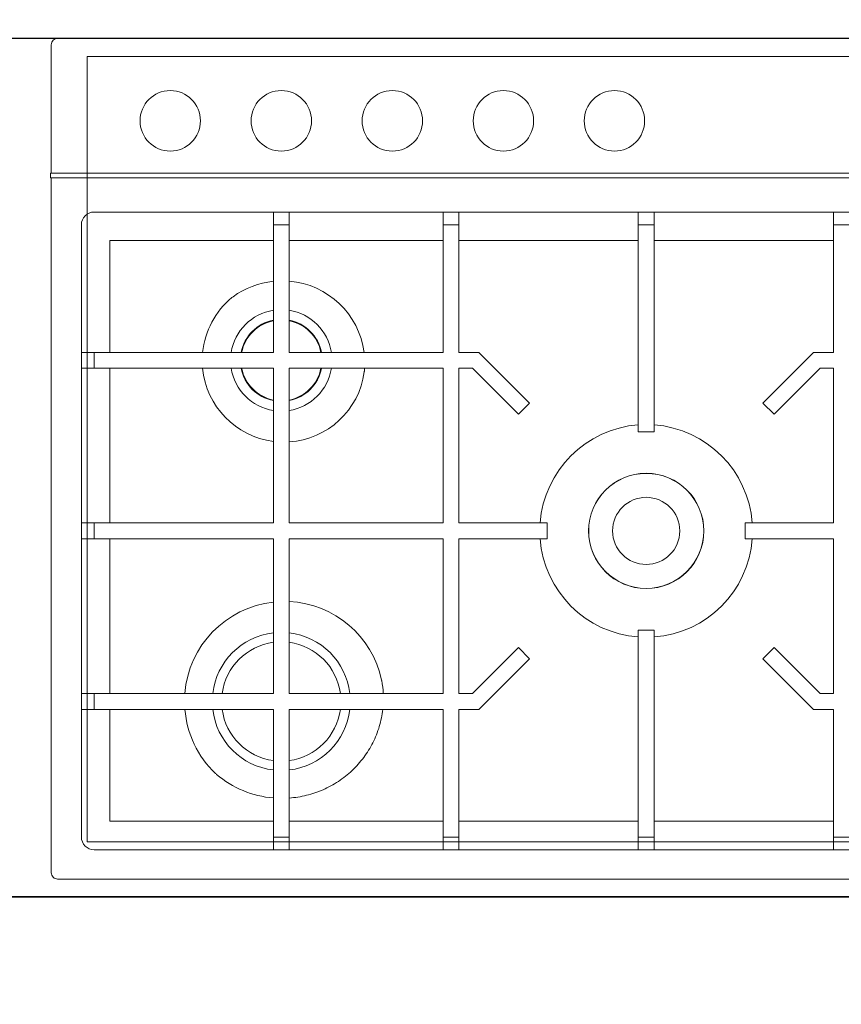
# Model space of a CAD drawing. Units: inches. Extents: x -1198 to -69, y -512 to 437.
# Tile 30 of 50: x -658 to -635, y 158 to 186. Entities that reach past the tile are written whole.
import ezdxf

# ---------------------------------------------------------------- set-up
doc = ezdxf.new("R2010")
doc.units = ezdxf.units.IN
doc.header["$MEASUREMENT"] = 0
for name, color, linetype, lineweight in [('0_Pen_No__7', 7, 'Continuous', 18), ('A-ANNO-DIMS', 2, 'Continuous', 18), ('A-EQPM', 60, 'Continuous', 18), ('A-FLOR-CASE', 7, 'Continuous', 25), ('A-WALL', 7, 'Continuous', 35)]:
    doc.layers.add(name, color=color, linetype=linetype, lineweight=lineweight)
doc.styles.get("Standard").update_dxf_attribs({"font": 'arial.ttf'})
doc.dimstyles.get("Standard").update_dxf_attribs({"dimtxt": 6, "dimasz": 6, "dimexe": 0.18, "dimexo": 0.0625, "dimgap": 0.09, "dimtad": 0, "dimtih": 1, "dimtoh": 1, "dimdec": 0, "dimzin": 0, "dimdsep": 46, "dimlunit": 4, "dimtxsty": 'Standard', "dimblk": 'OBLIQUE', "dimcen": 0.09, "dimadec": 0, "dimazin": 0, "dimtfac": 1, "dimtdec": 0, "dimtofl": 0, "dimtmove": 0, "dimatfit": 3, "dimfxl": 1, "dimtolj": 1, "dimtzin": 0, "dimarcsym": 0})

# ---------------------------------------------------------------- blocks, each defined once
blk = doc.blocks.new('new block')
at = {"layer": '0_Pen_No__7'}
for p, q in [((-80.82, 567.06), (-69.55, 567.06)), ((68.97, 567.06), (57.71, 567.06)), ((207.5, 567.06), (196.24, 567.06)), ((328.01, 567.06), (316.75, 567.06)), ((-69.55, 555.8), (57.71, 555.8)), ((196.24, 555.8), (68.97, 555.8)), ((316.75, 555.8), (207.5, 555.8)), ((444.01, 555.8), (328.01, 555.8)), ((444.01, 476.4), (444.01, 555.8)), ((455.27, 465.14), (455.27, 476.4)), ((444.01, 355.33), (444.01, 465.14)), ((455.27, 344.07), (455.27, 355.33)), ((444.01, 344.07), (444.01, 234.26)), ((455.27, 234.26), (455.27, 223)), ((-69.55, 143.6), (57.71, 143.6)), ((196.24, 143.6), (68.97, 143.6)), ((316.75, 143.6), (207.5, 143.6)), ((-80.82, 132.33), (-69.55, 132.33)), ((57.71, 132.33), (68.97, 132.33)), ((207.5, 132.33), (196.24, 132.33)), ((328.01, 132.33), (316.75, 132.33)), ((-359, 99.11), (485.68, 99.11)), ((485.68, 95.73), (-359, 95.73))]:
    blk.add_line(p, q, dxfattribs=at)
for points in [[(-354.49, 596.91), (481.18, 596.91, -0.414214), (485.68, 592.4), (485.68, 99.11), (486.24, 99.11), (486.24, 95.73), (485.68, 95.73), (485.68, 4.5, -0.414214), (481.18, 0), (-354.49, 0, -0.414214), (-359, 4.5), (-359, 95.73), (-359.56, 95.73), (-359.56, 99.11), (-359, 99.11), (-359, 592.4, -0.414214)], [(464.28, 132.33), (464.28, 567.06, 0.414214), (455.27, 576.07), (-328.59, 576.07, 0.414214), (-337.6, 567.06), (-337.6, 132.33, 0.414214), (-328.59, 123.32), (455.27, 123.32, 0.414214)]]:
    blk.add_lwpolyline(points, format="xyb", close=True, dxfattribs=at)
for points in [[(-69.55, 576.07), (-69.55, 476.4), (-55.4, 476.4), (-19.45, 440.45), (-27.41, 432.48), (-60.06, 465.14), (-69.55, 465.14), (-69.55, 355.33), (-7.05, 355.33), (-7.05, 344.07), (-69.55, 344.07), (-69.55, 234.26), (-60.06, 234.26), (-27.41, 266.91), (-19.45, 258.94), (-55.4, 223), (-69.55, 223), (-69.55, 123.32)], [(57.71, 576.07), (57.71, 420.09), (68.97, 420.09), (68.97, 576.07)], [(196.24, 123.32), (196.24, 223), (182.08, 223), (146.13, 258.94), (154.09, 266.91), (186.75, 234.26), (196.24, 234.26), (196.24, 344.07), (133.73, 344.07), (133.73, 355.33), (196.24, 355.33), (196.24, 465.14), (186.75, 465.14), (154.09, 432.48), (146.13, 440.45), (182.08, 476.4), (196.24, 476.4), (196.24, 576.07)], [(207.5, 576.07), (207.5, 476.4), (316.75, 476.4), (316.75, 576.07)], [(328.01, 576.07), (328.01, 476.4), (464.28, 476.4)], [(316.75, 539.36), (315.2, 539.23), (313.66, 539.07), (312.12, 538.88), (310.58, 538.65), (309.05, 538.4), (307.53, 538.1), (306.01, 537.78), (304.5, 537.42), (303, 537.04), (301.5, 536.62), (300.02, 536.16), (298.55, 535.68), (297.08, 535.17), (295.63, 534.62), (294.19, 534.05), (292.76, 533.44), (291.35, 532.8), (289.95, 532.14), (288.56, 531.44), (287.19, 530.71), (285.84, 529.96), (284.5, 529.18), (283.18, 528.36), (281.87, 527.52), (280.59, 526.66), (279.32, 525.76), (278.07, 524.84), (276.85, 523.89), (275.64, 522.92), (274.45, 521.92), (273.29, 520.89), (272.15, 519.84), (271.03, 518.76), (269.94, 517.67), (268.87, 516.54), (267.82, 515.4), (266.8, 514.23), (265.8, 513.04), (264.83, 511.83), (263.89, 510.6), (262.98, 509.35), (262.09, 508.08), (261.23, 506.78), (260.4, 505.47), (259.6, 504.15), (258.82, 502.8), (258.08, 501.44), (257.37, 500.06), (256.69, 498.67), (256.03, 497.26), (255.41, 495.84), (254.83, 494.41), (254.27, 492.96), (253.75, 491.5), (253.25, 490.03), (252.8, 488.55), (252.37, 487.05), (251.98, 485.55), (251.62, 484.04), (251.29, 482.53), (251, 481), (250.75, 479.47), (250.53, 477.94), (250.34, 476.4)], [(464.28, 465.14), (328.01, 465.14), (328.01, 355.33), (464.28, 355.33)], [(464.28, 234.26), (328.01, 234.26), (328.01, 344.07), (464.28, 344.07)], [(68.97, 123.32), (68.97, 279.31), (57.71, 279.31), (57.71, 123.32)], [(207.5, 123.32), (207.5, 223), (316.75, 223), (316.75, 123.32)], [(328.01, 123.32), (328.01, 223), (464.28, 223)], [(444.01, 223), (444.01, 143.6), (328.01, 143.6)]]:
    blk.add_lwpolyline(points, dxfattribs=at)
for points in [[(-333.7, 12.95), (460.3, 12.95), (460.3, 570.44), (-333.7, 570.44)], [(207.5, 465.14), (207.5, 355.33), (316.75, 355.33), (316.75, 465.14)], [(316.75, 234.26), (207.5, 234.26), (207.5, 344.07), (316.75, 344.07)]]:
    blk.add_lwpolyline(points, close=True, dxfattribs=at)
for centre, radius in [((63.34, 349.7), 40.95), ((63.34, 349.7), 40.83), ((63.34, 349.7), 23.84), ((85.87, 58.56), 21.45), ((164.7, 58.56), 21.45), ((243.54, 58.56), 21.45), ((322.38, 58.56), 21.45), ((401.21, 58.56), 21.45)]:
    blk.add_circle(centre, radius, dxfattribs=at)
for centre, radius, start, end in [((322.14, 468.12), 71.42, 49.7275, 85.28931), ((322.38, 470.77), 48.99, 96.60065, 173.39935), ((322.38, 470.77), 48.99, 6.60065, 83.39935), ((355.62, 507.66), 19.61, 46.47207, 49.65802), ((320.47, 470.71), 70.6, 4.62083, 46.44687), ((322.38, 470.77), 42.35, 97.64264, 172.3569), ((322.38, 470.77), 42.35, 7.6431, 82.35736), ((319.41, 468.81), 69.49, 183.03105, 190.60746), ((322.38, 470.77), 48.99, 186.60065, 263.39935), ((322.38, 470.77), 42.35, 187.6431, 262.35736), ((320.15, 470.72), 70.94, 276.3643, 355.48211), ((322.38, 470.77), 48.99, 276.60065, 353.39935), ((322.38, 470.77), 42.35, 277.64264, 352.3569), ((269.57, 459.48), 18.78, 190.60771, 191.88529), ((319.99, 470.1), 70.32, 191.89609, 267.35247), ((63.34, 349.7), 75.53, 94.27701, 175.72431), ((63.34, 349.7), 75.53, 4.27569, 85.72299), ((63.34, 349.7), 75.53, 184.27569, 265.72299), ((63.34, 349.7), 75.53, 274.27701, 355.72431), ((320.48, 229.1), 57.52, 93.72225, 172.22668), ((320.57, 228.68), 57.95, 5.52347, 82.62478), ((322.38, 228.63), 36.04, 98.99031, 171.00966), ((322.38, 228.63), 36.04, 8.99034, 81.00969), ((322.38, 228.63), 29.08, 101.17283, 168.8339), ((322.38, 228.63), 28.72, 101.31905, 168.69126), ((322.38, 228.63), 29.08, 11.1661, 78.82717), ((322.38, 228.63), 28.72, 11.30874, 78.68095), ((320.24, 230.21), 57.15, 173.81232, 175.93921), ((281.76, 234.38), 18.44, 172.21689, 173.81535), ((321.61, 230.78), 58.58, 187.63711, 265.23442), ((322.38, 228.63), 36.04, 188.99034, 261.00969), ((322.38, 228.63), 29.08, 191.1661, 258.82717), ((322.38, 228.63), 28.72, 191.30874, 258.68095), ((322.38, 228.63), 36.04, 278.99031, 351.00966), ((322.38, 228.63), 29.08, 281.17283, 348.8339), ((322.38, 228.63), 28.72, 281.31905, 348.69126), ((320.83, 228.69), 57.68, 309.3686, 354.33417), ((322.04, 230.74), 58.56, 275.84718, 306.13795), ((345.26, 198.93), 19.18, 306.17281, 309.34365)]:
    blk.add_arc(centre, radius, start, end, dxfattribs=at)
blk = doc.blocks.new('COUNTER-L')
at = {"ltscale": 10}
blk.add_line((49.349, 24), (0, 24), dxfattribs=at)
blk = doc.blocks.new('_Oblique')
at = {"color": 0, "linetype": 'ByBlock', "lineweight": -2}
blk.add_line((-0.5, -0.5), (0.5, 0.5), dxfattribs=at)
blk = doc.blocks.new('*D56')
at = {"layer": 'A-ANNO-DIMS', "color": 0, "lineweight": -2, "ltscale": 10, "transparency": 16777216}
for p, q in [((-618.339, 257.228), (-603.822, 257.228)), ((-604.002, 257.228), (-604.002, 212.422)), ((-604.002, 161.228), (-604.002, 206.033)), ((-618.339, 161.228), (-603.822, 161.228))]:
    blk.add_line(p, q, dxfattribs=at)
at = {"layer": 'DEFPOINTS', "color": 0, "ltscale": 10, "transparency": 16777216}
for p in [(-618.402, 257.228), (-604.002, 257.228), (-618.402, 161.228)]:
    blk.add_point(p, dxfattribs=at)
at = {"layer": 'A-ANNO-DIMS', "color": 0, "lineweight": -2, "ltscale": 10, "transparency": 16777216, "xscale": 6, "yscale": 6, "zscale": 6}
for p, rotation in [((-604.002, 257.228), 90), ((-604.002, 161.228), 270)]:
    blk.add_blockref('_Oblique', p, dxfattribs=dict(at, rotation=rotation))
at = {"layer": 'A-ANNO-DIMS', "color": 0, "ltscale": 10, "transparency": 16777216, "insert": (-604.002, 209.228), "char_height": 6, "attachment_point": 5}
blk.add_mtext('\\A1;COUNTER 96 TYP.', dxfattribs=at)
blk = doc.blocks.new('*D57')
at = {"layer": 'A-ANNO-DIMS', "color": 0, "lineweight": -2, "ltscale": 10, "transparency": 16777216}
for p, q in [((-667.751, 161.165), (-667.751, 146.648)), ((-618.402, 161.165), (-618.402, 146.648)), ((-667.751, 146.828), (-657.89, 146.828)), ((-618.402, 146.828), (-628.263, 146.828))]:
    blk.add_line(p, q, dxfattribs=at)
at = {"layer": 'DEFPOINTS', "color": 0, "ltscale": 10, "transparency": 16777216}
for p in [(-667.751, 161.228), (-618.402, 161.228), (-618.402, 146.828)]:
    blk.add_point(p, dxfattribs=at)
at = {"layer": 'A-ANNO-DIMS', "color": 0, "lineweight": -2, "ltscale": 10, "transparency": 16777216, "xscale": 6, "yscale": 6, "zscale": 6, "rotation": 180}
blk.add_blockref('_Oblique', (-667.751, 146.828), dxfattribs=at)
at = {"layer": 'A-ANNO-DIMS', "color": 0, "lineweight": -2, "ltscale": 10, "transparency": 16777216, "xscale": 6, "yscale": 6, "zscale": 6}
blk.add_blockref('_Oblique', (-618.402, 146.828), dxfattribs=at)
at = {"layer": 'A-ANNO-DIMS', "color": 0, "ltscale": 10, "transparency": 16777216, "insert": (-643.076, 146.828), "char_height": 6, "attachment_point": 5}
blk.add_mtext('\\A1;49 TYP.', dxfattribs=at)

msp = doc.modelspace()

# ---------------------------------------------------------------- linework, layer by layer
at = {"layer": 'A-WALL', "ltscale": 10}
msp.add_line((-565.7509, 161.2277), (-691.7509, 161.2277), dxfattribs=at)

# ---------------------------------------------------------------- block references
at = {"layer": 'A-EQPM', "xscale": 0.0393700787401575, "yscale": 0.0393700787401575, "zscale": 0.0393700787401575, "rotation": 180}
msp.add_blockref('new block', (-638.3186, 185.2277), dxfattribs=at)
at = {"layer": 'A-FLOR-CASE'}
msp.add_blockref('COUNTER-L', (-667.751, 161.228), dxfattribs=at)

# ---------------------------------------------------------------- dimensions: what is measured, and where the dimension line sits
at = {"layer": 'A-ANNO-DIMS', "ltscale": 10}
dim = msp.add_linear_dim(base=(-604.0019, 257.2277), p1=(-618.4019, 161.2277), p2=(-618.4019, 257.2277), angle=90, text='COUNTER <> TYP.', dimstyle='Standard', override={"dimdec": 0, "dimlfac": 1, "dimrnd": 0, "dimzin": 0, "dimdsep": 46, "dimlunit": 2}, dxfattribs=at)
dim.commit()
dim.dimension.update_dxf_attribs({"geometry": '*D56', "text_midpoint": (-604.0019, 209.2277)})
dim = msp.add_linear_dim(base=(-618.4019, 146.8277), p1=(-667.7509, 161.2277), p2=(-618.4019, 161.2277), text='<> TYP.', dimstyle='Standard', override={"dimdec": 0, "dimlfac": 1, "dimrnd": 0, "dimzin": 0, "dimdsep": 46, "dimlunit": 2}, dxfattribs=at)
dim.commit()
dim.dimension.update_dxf_attribs({"geometry": '*D57', "text_midpoint": (-643.0764, 146.8277)})

doc.saveas('drawing.dxf')
